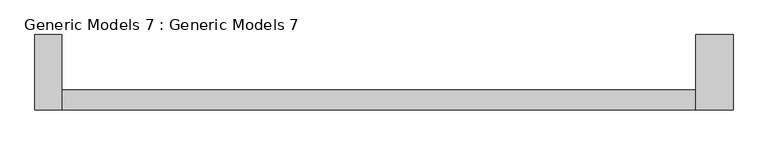
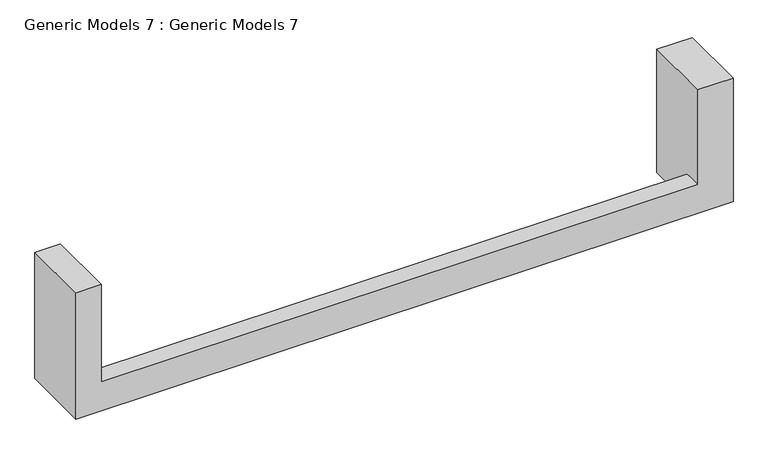
"""IFC4 building model written with IfcOpenShell, lengths in millimetres: proxy geometry, Generic Models 7 : Generic Models 7."""

from ifc_helpers import new_model, si_unit, origin, place, context, project, spatial, faceted_brep, source, transform, mapped, element, save


def generic_models_7_generic_models_7_06ca3c93(model_context):
    return source(origin(), model_context, "Body", "Brep", [
        faceted_brep([(-6626.0414575, -14658.1411535, 9753.6), (-12620.4414575, -14658.1411535, 9753.6), (-12620.4414575, -14845.9752569, 9753.6), (-6626.0414575, -14845.9752569, 9753.6), (-12620.4414575, -14658.1411535, 9448.8), (-6626.0414575, -14658.1411535, 9448.8), (-6626.0414575, -14134.7752569, 9448.8), (-6272.2195233, -14134.7752569, 9448.8), (-6272.2195233, -14845.9752569, 9448.8), (-12874.4414575, -14845.9752569, 9448.8), (-12874.4414575, -14134.7752569, 9448.8), (-12620.4414575, -14134.7752569, 9448.8), (-12620.4414575, -14845.9752569, 10790.5282636), (-12874.4414575, -14845.9752569, 10790.5282636), (-6272.2195233, -14845.9752569, 10762.4340464), (-6626.0414575, -14845.9752569, 10762.4340464), (-12620.4414575, -14134.7752569, 10790.5282636), (-12874.4414575, -14134.7752569, 10790.5282636), (-6626.0414575, -14134.7752569, 10762.4340464), (-6272.2195233, -14134.7752569, 10762.4340464)], [[[0, 1, 2, 3]], [[4, 5, 6, 7, 8, 9, 10, 11]], [[1, 0, 5, 4]], [[3, 2, 12, 13, 9, 8, 14, 15]], [[16, 17, 13, 12]], [[17, 16, 11, 10]], [[13, 17, 10, 9]], [[16, 12, 2, 1, 4, 11]], [[18, 15, 14, 19]], [[15, 18, 6, 5, 0, 3]], [[19, 14, 8, 7]], [[18, 19, 7, 6]]]),
    ])


if __name__ == "__main__":
    model = new_model("IFC4")
    model_context = context("Model", 3, world=origin())
    ifc_project = project(units=[si_unit("LENGTHUNIT", "METRE", prefix="MILLI")], contexts=[model_context])
    site = spatial("IfcSite", under=ifc_project)
    building = spatial("IfcBuilding", under=site)
    placement = place(None, origin())
    generic_models_7_generic_models_7_shape = generic_models_7_generic_models_7_06ca3c93(model_context)
    element("IfcBuildingElementProxy", 1, Name="Generic Models 7 : Generic Models 7", ObjectType="Generic Models 7 : Generic Models 7", at=placement, inside=building, context=model_context, shape_type="MappedRepresentation", body=[
        mapped(generic_models_7_generic_models_7_shape, transform((0.0, 0.0, 0.0), x_axis=(1.0, 0.0, 0.0), y_axis=(0.0, 1.0, 0.0), z_axis=(0.0, 0.0, 1.0))),
    ])
    save(model, "model.ifc")
